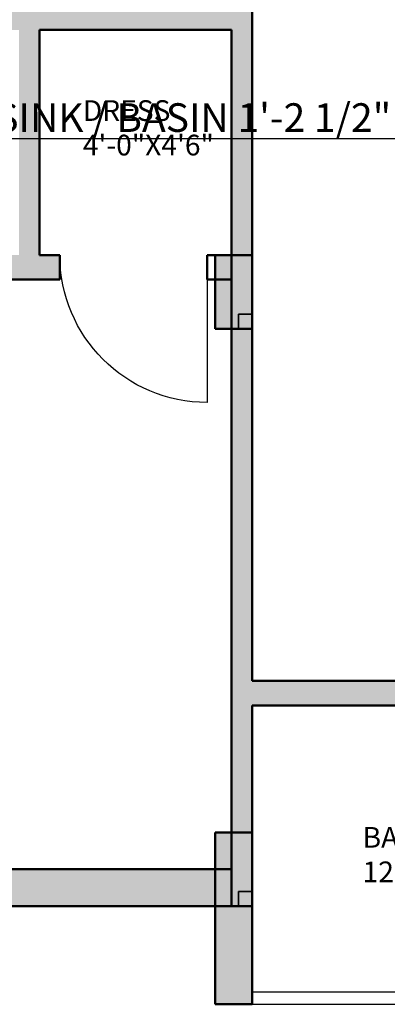
# Model space of a CAD drawing. Units: inches. Extents: x -7 to 1228, y -146 to 1091.
# Tile 6 of 88: x 179 to 269, y 36 to 276. Entities that reach past the tile are written whole.
import ezdxf

# ---------------------------------------------------------------- set-up
doc = ezdxf.new("R2010")
doc.units = ezdxf.units.IN
for name, color, linetype, lineweight in [('A-ANNO-DIMS', 2, 'Continuous', 18), ('A-AREA-IDEN', 7, 'Continuous', 18), ('A-COLS', 6, 'Continuous', 35), ('A-DOOR', 4, 'Continuous', 25), ('A-GLAZ', 175, 'Continuous', 25), ('A-WALL', 7, 'Continuous', 50), ('A-WALL-PATT', 251, 'Continuous', 13)]:
    doc.layers.add(name, color=color, linetype=linetype, lineweight=lineweight)
doc.styles.get("Standard").update_dxf_attribs({"font": 'arial.ttf'})
doc.dimstyles.new('ISO-25', dxfattribs={"dimtxt": 7, "dimasz": 4, "dimexe": 1.25, "dimexo": 0.625, "dimtad": 1, "dimdec": 1, "dimlunit": 3, "dimtxsty": 'Standard', "dimcen": 2.5, "dimadec": 0, "dimazin": 0, "dimtfac": 1, "dimtdec": 1, "dimtmove": 1, "dimatfit": 3, "dimfxl": 1, "dimarcsym": 0})

# ---------------------------------------------------------------- blocks, each defined once
blk = doc.blocks.new('DOOR-900')
blk.add_line((36, 0), (36, 36))
blk.add_arc((36, 0), 36, 90, 180)
blk = doc.blocks.new('*D32')
at = {"layer": 'A-ANNO-DIMS', "color": 0, "lineweight": -2, "transparency": 16777216}
for p, q in [((159.65, 262.03), (159.65, 259.24)), ((170.13, 260.49), (163.65, 260.49)), ((166.89, 260.49), (170.8, 247.44)), ((174.13, 262.03), (174.13, 259.24)), ((170.8, 247.44), (294.04, 247.44))]:
    blk.add_line(p, q, dxfattribs=at)
at = {"layer": 'A-ANNO-DIMS', "color": 0, "transparency": 16777216}
for points in [[(163.65, 261.15), (163.65, 259.82), (159.65, 260.49)], [(170.13, 261.15), (170.13, 259.82), (174.13, 260.49)]]:
    blk.add_solid(points, dxfattribs=at)
at = {"layer": 'Defpoints', "color": 0, "transparency": 16777216}
for p in [(159.65, 262.66), (174.13, 262.66), (159.65, 260.49)]:
    blk.add_point(p, dxfattribs=at)
at = {"layer": 'A-ANNO-DIMS', "color": 0, "transparency": 16777216, "insert": (232.42, 251.68), "char_height": 7, "attachment_point": 5}
blk.add_mtext('SINK / BASIN 1\'-2 1/2" TYP.', dxfattribs=at)

msp = doc.modelspace()

# ---------------------------------------------------------------- hatches: boundary and pattern name
at = {"layer": 'A-COLS'}
h = msp.add_hatch(color=256, dxfattribs=at)
h.dxf.hatch_style = 1
h.paths.add_polyline_path([(236, 219), (227, 219), (227, 201), (232.71, 201), (232.71, 204.55), (236, 204.55)])
h = msp.add_hatch(color=256, dxfattribs=at)
h.dxf.hatch_style = 1
h.paths.add_polyline_path([(232.71, 204.55), (232.71, 201), (236, 201), (236, 204.55)])
h = msp.add_hatch(color=256, dxfattribs=at)
h.dxf.hatch_style = 1
h.paths.add_polyline_path([(236, 78), (227, 78), (227, 60), (232.71, 60), (232.71, 63.55), (236, 63.55)])
h = msp.add_hatch(color=256, dxfattribs=at)
h.dxf.hatch_style = 1
h.paths.add_polyline_path([(232.71, 63.55), (232.71, 60), (236, 60), (236, 63.55)])
at = {"layer": 'A-WALL-PATT'}
h = msp.add_hatch(color=256, dxfattribs=at)
h.dxf.hatch_style = 1
h.paths.add_polyline_path([(69, 568), (60, 568), (60, 493), (63.29, 493), (69, 493)])
h.paths.add_polyline_path([(69, 662.41), (60, 662.41), (60, 586), (69, 586)], flags=17)
h.paths.add_polyline_path([(69, 723), (184, 723), (184, 734), (179, 734), (179, 728), (69, 728), (69, 741.62), (60, 741.62), (60, 698.41), (69, 698.41)], flags=17)
h.paths.add_polyline_path([(69, 782), (231, 782), (231, 728), (231, 723), (231, 586), (236, 586), (236, 787), (69, 787), (69, 800.13), (60, 800.13), (60, 765.62), (69, 765.62)])
h.paths.add_polyline_path([(184, 842), (189, 842), (189, 848), (173, 848), (173, 842), (179, 842), (179, 787), (184, 787)])
h.paths.add_polyline_path([(118.22, 69), (69, 69), (69, 60), (118.22, 60)])
h.paths.add_polyline_path([(227, 69), (154.22, 69), (154.22, 60), (227, 60)])
h.paths.add_polyline_path([(236, 60), (232.71, 60), (227, 60), (227, 36), (236, 36)])
h.paths.add_polyline_path([(389, 60), (380, 60), (380, 36), (389, 36)])
h.paths.add_polyline_path([(384, 181), (380, 181), (380, 115), (380, 78), (384, 78)])
h.paths.add_polyline_path([(380, 115), (334.55, 115), (334.55, 109), (380, 109)])
h.paths.add_polyline_path([(274.55, 115), (236, 115), (236, 201), (232.71, 201), (231, 201), (231, 78), (236, 78), (236, 109), (274.55, 109)])
h.paths.add_polyline_path([(69, 123), (60, 123), (60, 78), (69, 78)])
h.paths.add_polyline_path([(69, 201), (60, 201), (60, 159), (69, 159)])
h.paths.add_polyline_path([(143, 219), (69, 219), (69, 213), (143, 213)], flags=17)
h.paths.add_polyline_path([(189, 219), (184, 219), (184, 274), (231, 274), (231, 219), (236, 219), (236, 279), (184, 279), (184, 297), (179, 297), (179, 279), (69, 279), (69, 290.91), (60, 290.91), (60, 262.18), (69, 262.18), (69, 274), (179, 274), (179, 219), (173, 219), (173, 213), (189, 213)])
h.paths.add_polyline_path([(69, 238.18), (60, 238.18), (60, 219), (69, 219)], flags=17)
h.paths.add_polyline_path([(69, 333), (60, 333), (60, 314.91), (69, 314.91), (69, 316.96)])
h.paths.add_polyline_path([(190, 338), (184, 338), (69, 338), (69, 333), (179, 333), (179, 327), (184, 327), (184, 333.02), (190, 333.05)])
h.paths.add_polyline_path([(69, 386.81), (60, 386.81), (60, 351), (69, 351)])
h.paths.add_polyline_path([(69, 475), (60, 475), (60, 422.81), (69, 422.81)])
h.paths.add_polyline_path([(236, 475), (231, 475), (231, 351.24), (236, 351.24)])
h.paths.add_polyline_path([(384, 475), (380, 475), (380, 362), (384, 362)])
h.paths.add_polyline_path([(547, 307), (439, 307), (439, 356), (445, 356), (445, 362), (433, 362), (433, 307), (380, 307), (380, 244), (380, 241), (384, 241), (384, 301), (433, 301), (433, 277), (439, 277), (439, 301), (547, 301)])
h.paths.add_polyline_path([(547, 241), (439, 241), (439, 247), (433, 247), (433, 235), (547, 235)])
h.paths.add_polyline_path([(450, 69), (440.29, 69), (424.89, 69), (389, 69), (389, 60), (450, 60)])
h.paths.add_polyline_path([(547, 69), (486, 69), (486, 60), (547, 60)])
h.paths.add_polyline_path([(556, 148.27), (547, 148.27), (547, 78), (556, 78)])
h.paths.add_polyline_path([(556, 223), (547, 223), (547, 195), (547, 184.27), (556, 184.27)])
h.paths.add_polyline_path([(556, 311.19), (547, 311.19), (547, 273.08), (556, 273.08)])
h.paths.add_polyline_path([(556, 344), (552.71, 344), (547, 344), (547, 335.19), (556, 335.19)])
h.paths.add_polyline_path([(556, 249.08), (547, 249.08), (547, 241), (556, 241)])
h.paths.add_polyline_path([(547, 362), (475, 362), (475, 356), (547, 356)], flags=0)
h.paths.add_polyline_path([(556, 399.62), (547, 399.62), (547, 362), (556, 362)])
h.paths.add_polyline_path([(556, 475), (547, 475), (547, 435.62), (556, 435.62)])
h.paths.add_polyline_path([(547, 493), (389, 493), (389, 487), (547, 487)])
h.paths.add_polyline_path([(380, 493), (278, 493), (278, 487), (380, 487)])
h.paths.add_polyline_path([(227, 493), (69, 493), (69, 487), (227, 487)])
h.paths.add_polyline_path([(643, 122.44), (634, 122.44), (634, 78), (643, 78)])
h.paths.add_polyline_path([(702.5, 69), (692.79, 69), (677.39, 69), (643, 69), (643, 60), (702.5, 60)])
h.paths.add_polyline_path([(798, 69), (738.5, 69), (738.5, 60), (798, 60)])
h.paths.add_polyline_path([(807, 60), (803.71, 60), (798, 60), (798, 36), (807, 36)])
h.paths.add_polyline_path([(807, 109), (846.75, 109), (846.75, 115), (807, 115), (807, 159), (802, 159), (802, 78), (807, 78)])
h.paths.add_polyline_path([(807, 201), (802, 201), (802, 195), (807, 195)])
h.paths.add_polyline_path([(643, 201), (634, 201), (634, 158.44), (643, 158.44)])
h.paths.add_polyline_path([(756, 225), (751, 225), (751, 219), (643, 219), (643, 213), (756, 213)])
h.paths.add_polyline_path([(643, 240.85), (634, 240.85), (634, 219), (643, 219)])
h.paths.add_polyline_path([(643, 274), (643, 288.63), (634, 288.63), (634, 264.85), (643, 264.85)])
h.paths.add_polyline_path([(802, 279), (756, 279), (756, 297), (751, 297), (751, 279), (643, 279), (643, 274), (751, 274), (751, 255), (756, 255), (756, 274), (802, 274)])
h.paths.add_polyline_path([(807, 333), (803.71, 333), (802, 333), (802, 279), (802, 274), (802, 219), (807, 219)])
h.paths.add_polyline_path([(956, 182), (951, 182), (951, 115), (906.75, 115), (906.75, 109), (951, 109), (951, 78), (956, 78)])
h.paths.add_polyline_path([(960, 60), (951, 60), (951, 36), (960, 36)])
h.paths.add_polyline_path([(1021, 69), (1005.78, 69), (960, 69), (960, 60), (1021, 60)])
h.paths.add_polyline_path([(956, 224), (951, 224), (951, 218), (956, 218)])
h.paths.add_polyline_path([(956, 302), (1004, 302), (1004, 278), (1010, 278), (1010, 302), (1118, 302), (1118, 290.81), (1127, 290.81), (1127, 326.97), (1118, 326.97), (1118, 320.97), (1118, 307), (1010, 307), (1010, 356), (1016, 356), (1016, 362), (1004, 362), (1004, 307), (951, 307), (951, 244), (951, 242), (954.29, 242), (956, 242)])
h.paths.add_polyline_path([(643, 333), (634, 333), (634, 312.63), (643, 312.63), (643, 316.96)])
h.paths.add_polyline_path([(756, 338), (643, 338), (643, 333), (751, 333), (751, 327), (756, 327)])
h.paths.add_polyline_path([(643, 388), (634, 388), (634, 351), (643, 351)])
h.paths.add_polyline_path([(807, 357), (802, 357), (802, 351), (807, 351)])
h.paths.add_polyline_path([(807, 475), (802, 475), (802, 393), (807, 393)])
h.paths.add_polyline_path([(643, 475), (634, 475), (634, 424), (643, 424)])
h.paths.add_polyline_path([(798, 493), (643, 493), (643, 487), (798, 487)])
h.paths.add_polyline_path([(634, 493), (556, 493), (556, 487), (634, 487)])
h.paths.add_polyline_path([(813, 493), (807, 493), (807, 487), (813, 487)])
h.paths.add_polyline_path([(951, 493), (849, 493), (849, 487), (951, 487)])
h.paths.add_polyline_path([(956, 484), (951, 484), (951, 374), (956, 374)])
h.paths.add_polyline_path([(1109, 493), (969, 493), (969, 487), (1109, 487)])
h.paths.add_polyline_path([(1127, 484), (1118, 484), (1118, 450.64), (1127, 450.64)])
h.paths.add_polyline_path([(1127, 414.64), (1118, 414.64), (1118, 365), (1127, 365)])
h.paths.add_polyline_path([(1109, 362), (1046, 362), (1046, 356), (1109, 356)], flags=17)
h.paths.add_polyline_path([(1127, 356), (1123.45, 356), (1118, 356), (1118, 350.97), (1127, 350.97)], flags=0)
h.paths.add_polyline_path([(1127, 266.81), (1118, 266.81), (1118, 262.36), (1118, 242), (1127, 242)], flags=17)
h.paths.add_polyline_path([(1118, 242), (1010, 242), (1010, 248), (1004, 248), (1004, 237), (1118, 237)])
h.paths.add_polyline_path([(1127, 224), (1118, 224), (1118, 170), (1127, 170)])
h.paths.add_polyline_path([(1127, 134), (1118, 134), (1118, 78), (1127, 78)])
h.paths.add_polyline_path([(1118, 69), (1057, 69), (1057, 60), (1118, 60)])
h.paths.add_polyline_path([(227, 571.55), (227, 574), (69, 574), (69, 568), (227, 568)])
h.paths.add_polyline_path([(380, 571.55), (380, 574), (278, 574), (278, 568), (380, 568)])
h.paths.add_polyline_path([(242, 574), (236, 574), (236, 568), (242, 568)])
h.paths.add_polyline_path([(547, 571.55), (547, 574), (389, 574), (389, 568), (547, 568)])
h.paths.add_polyline_path([(384, 733), (380, 733), (380, 586), (384, 586)])
h.paths.add_polyline_path([(556, 646), (634, 646), (634, 655), (547, 655), (547, 586), (556, 586)])
h.paths.add_polyline_path([(634, 574), (556, 574), (556, 568), (634, 568)])
h.paths.add_polyline_path([(643, 655), (634, 655), (634, 586), (643, 586)])
h.paths.add_polyline_path([(798, 574), (643, 574), (643, 568), (798, 568)])
h.paths.add_polyline_path([(643, 663.85), (634, 663.85), (634, 655), (643, 655)])
h.paths.add_polyline_path([(556, 676.97), (547, 676.97), (547, 655), (556, 655)])
h.paths.add_polyline_path([(556, 733), (547, 733), (547, 712.97), (556, 712.97)])
h.paths.add_polyline_path([(643, 710), (634, 710), (634, 699.85), (643, 699.85)])
h.paths.add_polyline_path([(807, 668), (802, 668), (802, 586), (807, 586)])
h.paths.add_polyline_path([(951, 574), (849, 574), (849, 568), (951, 568)])
h.paths.add_polyline_path([(956, 691), (951, 691), (951, 577), (956, 577)])
h.paths.add_polyline_path([(1109, 574), (969, 574), (969, 568), (1109, 568)])
h.paths.add_polyline_path([(1127, 643.4), (1118, 643.4), (1118, 577), (1127, 577)])
h.paths.add_polyline_path([(1127, 568), (1123.45, 568), (1118, 568), (1118, 493), (1127, 493)])
h.paths.add_polyline_path([(1127, 733), (1118, 733), (1118, 679.4), (1127, 679.4)])
h.paths.add_polyline_path([(1127, 777.35), (1118, 777.35), (1118, 770.04), (1118, 751), (1127, 751)], flags=17)
h.paths.add_polyline_path([(1118, 751), (1010, 751), (1010, 757), (1004, 757), (1004, 745), (1118, 745)])
h.paths.add_polyline_path([(956, 811), (1004, 811), (1004, 787), (1010, 787), (1010, 811), (1017.87, 811), (1017.87, 811.63, -0.414214), (1018.25, 812), (1031.98, 812, -0.414214), (1032.35, 811.63), (1032.35, 811), (1118, 811), (1118, 801.35), (1127, 801.35), (1127, 834.69), (1118, 834.69), (1118, 830.24), (1118, 817), (1010, 817), (1010, 866), (1016, 866), (1016, 872), (1004, 872), (1004, 817), (956, 817), (956, 866), (951, 866), (951, 751), (954.29, 751), (956, 751)])
h.paths.add_polyline_path([(1118, 872), (1046, 872), (1046, 866), (1118, 866)], flags=17)
h.paths.add_polyline_path([(1127, 924.71), (1118, 924.71), (1118, 884), (1127, 884)])
h.paths.add_polyline_path([(1127, 866), (1123.71, 866), (1118, 866), (1118, 858.69), (1127, 858.69)], flags=17)
h.paths.add_polyline_path([(956, 983), (951, 983), (951, 952), (807, 952), (807, 983), (802, 983), (802, 902), (807, 902), (807, 946), (951, 946), (951, 884), (956, 884)])
h.paths.add_polyline_path([(807, 842), (802, 842), (802, 787), (756, 787), (756, 806), (751, 806), (751, 787), (643, 787), (643, 782), (751, 782), (751, 764), (756, 764), (756, 782), (802, 782), (802, 728), (807, 728)])
h.paths.add_polyline_path([(756, 848), (643, 848), (643, 842), (751, 842), (751, 836), (756, 836)])
h.paths.add_polyline_path([(756, 734), (751, 734), (751, 728), (643, 728), (643, 723), (756, 723)])
h.paths.add_polyline_path([(643, 749.79), (634, 749.79), (634, 728), (637.29, 728), (643, 728)])
h.paths.add_polyline_path([(643, 805.41), (634, 805.41), (634, 773.79), (643, 773.79)])
h.paths.add_polyline_path([(643, 896.66), (634, 896.66), (634, 860), (637.29, 860), (643, 860)])
h.paths.add_polyline_path([(643, 842), (634, 842), (634, 829.41), (643, 829.41)])
h.paths.add_polyline_path([(643, 983), (634, 983), (634, 932.66), (643, 932.66)])
h.paths.add_polyline_path([(1127, 983), (1118, 983), (1118, 960.71), (1127, 960.71)])
h.paths.add_polyline_path([(1118, 1001), (1077.53, 1001), (1077.53, 992), (1118, 992)])
h.paths.add_polyline_path([(1041.53, 1001), (960, 1001), (960, 992), (1041.53, 992)])
h.paths.add_polyline_path([(960, 1025), (951, 1025), (951, 1001), (954.29, 1001), (960, 1001)])
h.paths.add_polyline_path([(807, 1025), (798, 1025), (798, 1001), (807, 1001)])
h.paths.add_polyline_path([(798, 1001), (738.5, 1001), (738.5, 992), (798, 992)])
h.paths.add_polyline_path([(702.5, 1001), (643, 1001), (643, 992), (702.5, 992)])
h.paths.add_polyline_path([(547, 1001), (499.11, 1001), (499.11, 992), (547, 992)])
h.paths.add_polyline_path([(463.11, 1001), (389, 1001), (389, 992), (463.11, 992)])
h.paths.add_polyline_path([(389, 1025), (380, 1025), (380, 1022), (380, 1001), (383.29, 1001), (389, 1001)])
h.paths.add_polyline_path([(236, 1025), (227, 1025), (227, 1001), (236, 1001)])
h.paths.add_polyline_path([(236, 983), (231, 983), (231, 860), (236, 860)])
h.paths.add_polyline_path([(274.55, 952), (236, 952), (236, 946), (274.55, 946)])
h.paths.add_polyline_path([(380, 952), (334.55, 952), (334.55, 946), (380, 946)])
h.paths.add_polyline_path([(384, 983), (380, 983), (380, 884), (383.29, 884), (384, 884)])
h.paths.add_polyline_path([(227, 1001), (155.01, 1001), (155.01, 992), (162.87, 992), (227, 992)])
h.paths.add_polyline_path([(119.01, 1001), (69, 1001), (69, 992), (119.01, 992)])
h.paths.add_polyline_path([(69, 983), (60, 983), (60, 922.99), (69, 922.99)])
h.paths.add_polyline_path([(69, 886.99), (60, 886.99), (60, 860), (63.29, 860), (69, 860)])
h.paths.add_polyline_path([(143, 848), (69, 848), (69, 842), (143, 842)])

# ---------------------------------------------------------------- linework, layer by layer
at = {"layer": 'A-COLS'}
for points in [[(236, 201), (232.71, 201), (232.71, 204.55), (236, 204.55)], [(236, 60), (232.71, 60), (232.71, 63.55), (236, 63.55)]]:
    msp.add_lwpolyline(points, close=True, dxfattribs=at)
at = {"layer": 'A-GLAZ'}
for p, q in [((380, 39), (236, 39)), ((236, 36), (380, 36))]:
    msp.add_line(p, q, dxfattribs=at)
at = {"layer": 'A-WALL'}
for p, q in [((236, 274), (236, 279)), ((236, 279), (236, 115)), ((231, 274), (184, 274)), ((184, 219), (184, 274)), ((231, 274), (231, 60)), ((189, 219), (184, 219)), ((189, 219), (189, 213)), ((236, 219), (225, 219)), ((225, 213), (225, 219)), ((227, 201), (227, 219)), ((227, 219), (236, 219)), ((236, 219), (236, 201)), ((236, 115), (236, 219)), ((189, 213), (173, 213)), ((231, 213), (225, 213)), ((231, 69), (231, 213)), ((236, 201), (227, 201)), ((380, 115), (236, 115)), ((236, 69), (236, 109)), ((380, 109), (236, 109)), ((236, 109), (236, 60)), ((227, 60), (227, 78)), ((227, 78), (236, 78)), ((236, 78), (236, 60)), ((231, 69), (69, 69)), ((227, 36), (227, 69)), ((236, 69), (236, 60)), ((60, 60), (236, 60)), ((236, 60), (60, 60)), ((236, 60), (227, 60)), ((236, 60), (236, 60)), ((236, 60), (236, 36)), ((236, 36), (227, 36))]:
    msp.add_line(p, q, dxfattribs=at)

# ---------------------------------------------------------------- block references
at = {"layer": 'A-DOOR', "extrusion": (0, 0, -1), "zscale": -1, "rotation": 180}
msp.add_blockref('DOOR-900', (-189, 219), dxfattribs=at)

# ---------------------------------------------------------------- texts
at = {"layer": 'A-AREA-IDEN', "attachment_point": 1}
for s, insert, char_height in [('DRESS\\P4\'-0"X4\'6"', (194.62, 256.83), 5.057), ('BALCONY\\P12\'-0"X5\'-10"', (263.01, 79.31), 5.0568)]:
    msp.add_mtext_dynamic_manual_height_columns(s, width=137.2821, gutter_width=25.28, heights=[0], dxfattribs=dict(at, insert=insert, char_height=char_height))

# ---------------------------------------------------------------- dimensions: what is measured, and where the dimension line sits
at = {"layer": 'A-ANNO-DIMS'}
dim = msp.add_linear_dim(base=(159.65, 260.49), p1=(174.13, 262.66), p2=(159.65, 262.66), angle=180, text='SINK / BASIN <> TYP.', dimstyle='ISO-25', override={"dimdec": 1, "dimlfac": 1, "dimrnd": 0, "dimzin": 1, "dimdsep": 46, "dimlunit": 4, "dimfrac": 2}, dxfattribs=at)
dim.commit()
dim.dimension.update_dxf_attribs({"geometry": '*D32', "text_midpoint": (171.43, 251.68)})

doc.saveas('drawing.dxf')
